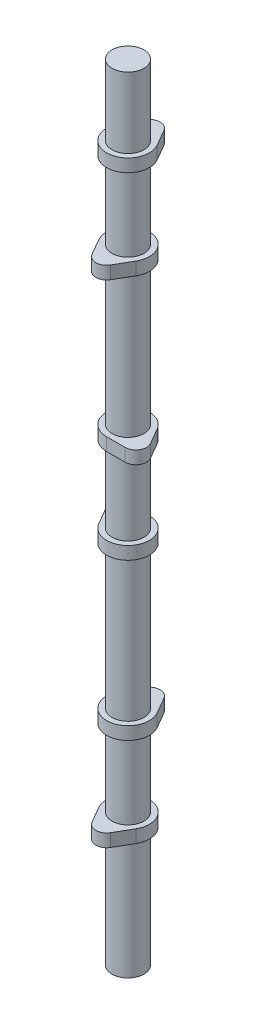
ISO-10303-21;
HEADER;
FILE_DESCRIPTION(('STEP AP214'),'2;1');
FILE_NAME('part.step','',(''),(''),'','','');
FILE_SCHEMA(('AUTOMOTIVE_DESIGN { 1 0 10303 214 1 1 1 1 }'));
ENDSEC;
DATA;
#1=APPLICATION_CONTEXT('core data for automotive mechanical design processes');
#2=APPLICATION_PROTOCOL_DEFINITION('international standard','automotive_design',2000,#1);
#3=PRODUCT_CONTEXT('',#1,'mechanical');
#4=PRODUCT('Part','Part','',(#3));
#5=PRODUCT_RELATED_PRODUCT_CATEGORY('part','',(#4));
#6=PRODUCT_DEFINITION_FORMATION('','',#4);
#7=PRODUCT_DEFINITION_CONTEXT('part definition',#1,'design');
#8=PRODUCT_DEFINITION('design','',#6,#7);
#9=PRODUCT_DEFINITION_SHAPE('','',#8);
#10=(LENGTH_UNIT() NAMED_UNIT(*) SI_UNIT(.MILLI.,.METRE.));
#11=(NAMED_UNIT(*) PLANE_ANGLE_UNIT() SI_UNIT($,.RADIAN.));
#12=(NAMED_UNIT(*) SI_UNIT($,.STERADIAN.) SOLID_ANGLE_UNIT());
#13=UNCERTAINTY_MEASURE_WITH_UNIT(LENGTH_MEASURE(1.E-05),#10,'distance_accuracy_value','');
#14=(GEOMETRIC_REPRESENTATION_CONTEXT(3) GLOBAL_UNCERTAINTY_ASSIGNED_CONTEXT((#13)) GLOBAL_UNIT_ASSIGNED_CONTEXT((#10,
#11,#12)) REPRESENTATION_CONTEXT('',''));
#15=CARTESIAN_POINT('',(0.,0.,0.));
#16=DIRECTION('',(0.,0.,1.));
#17=DIRECTION('',(1.,0.,0.));
#18=AXIS2_PLACEMENT_3D('',#15,#16,#17);
#19=CARTESIAN_POINT('',(0.,7.62,-12.7));
#20=DIRECTION('',(0.,-1.,0.));
#21=DIRECTION('',(0.,0.,-1.));
#22=AXIS2_PLACEMENT_3D('',#19,#20,#21);
#23=CYLINDRICAL_SURFACE('',#22,6.35);
#24=CARTESIAN_POINT('',(0.,0.,-12.7));
#25=DIRECTION('',(0.,1.,0.));
#26=DIRECTION('',(0.,0.,1.));
#27=AXIS2_PLACEMENT_3D('',#24,#25,#26);
#28=CIRCLE('',#27,6.35);
#29=CARTESIAN_POINT('',(5.49926131403118,0.,-15.875));
#30=VERTEX_POINT('',#29);
#31=CARTESIAN_POINT('',(-5.49926131403118,0.,-15.875));
#32=VERTEX_POINT('',#31);
#33=EDGE_CURVE('E384',#30,#32,#28,.T.);
#34=ORIENTED_EDGE('',*,*,#33,.T.);
#35=DIRECTION('',(0.,-1.,0.));
#36=VECTOR('',#35,1.);
#37=CARTESIAN_POINT('',(-5.49926131403118,7.62,-15.875));
#38=LINE('',#37,#36);
#39=CARTESIAN_POINT('',(-5.49926131403118,7.62,-15.875));
#40=VERTEX_POINT('',#39);
#41=EDGE_CURVE('E380',#40,#32,#38,.T.);
#42=ORIENTED_EDGE('',*,*,#41,.F.);
#43=CARTESIAN_POINT('',(0.,7.62,-12.7));
#44=DIRECTION('',(0.,1.,0.));
#45=DIRECTION('',(0.,0.,1.));
#46=AXIS2_PLACEMENT_3D('',#43,#44,#45);
#47=CIRCLE('',#46,6.35);
#48=CARTESIAN_POINT('',(5.49926131403118,7.62,-15.875));
#49=VERTEX_POINT('',#48);
#50=EDGE_CURVE('E378',#49,#40,#47,.T.);
#51=ORIENTED_EDGE('',*,*,#50,.F.);
#52=DIRECTION('',(0.,-1.,0.));
#53=VECTOR('',#52,1.);
#54=CARTESIAN_POINT('',(5.49926131403118,7.62,-15.875));
#55=LINE('',#54,#53);
#56=EDGE_CURVE('E383',#49,#30,#55,.T.);
#57=ORIENTED_EDGE('',*,*,#56,.T.);
#58=EDGE_LOOP('',(#34,#42,#51,#57));
#59=FACE_BOUND('',#58,.T.);
#60=ADVANCED_FACE('F39',(#59),#23,.T.);
#61=CARTESIAN_POINT('',(-5.49926131403118,7.62,-15.875));
#62=DIRECTION('',(0.866025403784438,0.,0.5));
#63=DIRECTION('',(0.5,0.,-0.866025403784439));
#64=AXIS2_PLACEMENT_3D('',#61,#62,#63);
#65=PLANE('',#64);
#66=DIRECTION('',(-0.5,0.,0.866025403784439));
#67=VECTOR('',#66,1.);
#68=CARTESIAN_POINT('',(-5.49926131403118,0.,-15.875));
#69=LINE('',#68,#67);
#70=CARTESIAN_POINT('',(-10.9985226280624,0.,-6.35));
#71=VERTEX_POINT('',#70);
#72=EDGE_CURVE('E389',#32,#71,#69,.T.);
#73=ORIENTED_EDGE('',*,*,#72,.T.);
#74=DIRECTION('',(0.,-1.,0.));
#75=VECTOR('',#74,1.);
#76=CARTESIAN_POINT('',(-10.9985226280624,7.62,-6.35));
#77=LINE('',#76,#75);
#78=CARTESIAN_POINT('',(-10.9985226280624,7.62,-6.35));
#79=VERTEX_POINT('',#78);
#80=EDGE_CURVE('E392',#79,#71,#77,.T.);
#81=ORIENTED_EDGE('',*,*,#80,.F.);
#82=DIRECTION('',(-0.5,0.,0.866025403784439));
#83=VECTOR('',#82,1.);
#84=CARTESIAN_POINT('',(-5.49926131403118,7.62,-15.875));
#85=LINE('',#84,#83);
#86=EDGE_CURVE('E87',#40,#79,#85,.T.);
#87=ORIENTED_EDGE('',*,*,#86,.F.);
#88=ORIENTED_EDGE('',*,*,#41,.T.);
#89=EDGE_LOOP('',(#73,#81,#87,#88));
#90=FACE_BOUND('',#89,.T.);
#91=ADVANCED_FACE('F464',(#90),#65,.F.);
#92=CARTESIAN_POINT('',(0.,7.62,0.));
#93=DIRECTION('',(0.,-1.,0.));
#94=DIRECTION('',(0.,0.,-1.));
#95=AXIS2_PLACEMENT_3D('',#92,#93,#94);
#96=CYLINDRICAL_SURFACE('',#95,12.7);
#97=CARTESIAN_POINT('',(0.,0.,0.));
#98=DIRECTION('',(0.,1.,0.));
#99=DIRECTION('',(0.,0.,1.));
#100=AXIS2_PLACEMENT_3D('',#97,#98,#99);
#101=CIRCLE('',#100,12.7);
#102=CARTESIAN_POINT('',(10.9985226280624,0.,-6.35));
#103=VERTEX_POINT('',#102);
#104=EDGE_CURVE('E71',#71,#103,#101,.T.);
#105=ORIENTED_EDGE('',*,*,#104,.T.);
#106=DIRECTION('',(0.,-1.,0.));
#107=VECTOR('',#106,1.);
#108=CARTESIAN_POINT('',(10.9985226280624,7.62,-6.35));
#109=LINE('',#108,#107);
#110=CARTESIAN_POINT('',(10.9985226280624,7.62,-6.35));
#111=VERTEX_POINT('',#110);
#112=EDGE_CURVE('E391',#111,#103,#109,.T.);
#113=ORIENTED_EDGE('',*,*,#112,.F.);
#114=CARTESIAN_POINT('',(0.,7.62,0.));
#115=DIRECTION('',(0.,1.,0.));
#116=DIRECTION('',(0.,0.,1.));
#117=AXIS2_PLACEMENT_3D('',#114,#115,#116);
#118=CIRCLE('',#117,12.7);
#119=EDGE_CURVE('E381',#79,#111,#118,.T.);
#120=ORIENTED_EDGE('',*,*,#119,.F.);
#121=ORIENTED_EDGE('',*,*,#80,.T.);
#122=EDGE_LOOP('',(#105,#113,#120,#121));
#123=FACE_BOUND('',#122,.T.);
#124=ADVANCED_FACE('F466',(#123),#96,.T.);
#125=CARTESIAN_POINT('',(5.49926131403118,7.62,-15.875));
#126=DIRECTION('',(-0.866025403784438,0.,0.5));
#127=DIRECTION('',(0.5,0.,0.866025403784439));
#128=AXIS2_PLACEMENT_3D('',#125,#126,#127);
#129=PLANE('',#128);
#130=DIRECTION('',(-0.5,0.,-0.866025403784439));
#131=VECTOR('',#130,1.);
#132=CARTESIAN_POINT('',(5.49926131403118,0.,-15.875));
#133=LINE('',#132,#131);
#134=EDGE_CURVE('E79',#103,#30,#133,.T.);
#135=ORIENTED_EDGE('',*,*,#134,.T.);
#136=ORIENTED_EDGE('',*,*,#56,.F.);
#137=DIRECTION('',(-0.5,0.,-0.866025403784439));
#138=VECTOR('',#137,1.);
#139=CARTESIAN_POINT('',(5.49926131403118,7.62,-15.875));
#140=LINE('',#139,#138);
#141=EDGE_CURVE('E54',#111,#49,#140,.T.);
#142=ORIENTED_EDGE('',*,*,#141,.F.);
#143=ORIENTED_EDGE('',*,*,#112,.T.);
#144=EDGE_LOOP('',(#135,#136,#142,#143));
#145=FACE_BOUND('',#144,.T.);
#146=ADVANCED_FACE('F476',(#145),#129,.F.);
#147=CARTESIAN_POINT('',(0.,7.62,-12.7));
#148=DIRECTION('',(0.,1.,0.));
#149=DIRECTION('',(0.,0.,1.));
#150=AXIS2_PLACEMENT_3D('',#147,#148,#149);
#151=PLANE('',#150);
#152=CARTESIAN_POINT('',(0.,7.62000000000002,0.));
#153=DIRECTION('',(0.,1.,0.));
#154=DIRECTION('',(0.,0.,1.));
#155=AXIS2_PLACEMENT_3D('',#152,#153,#154);
#156=CIRCLE('',#155,9.5);
#157=CARTESIAN_POINT('',(0.,7.62000000000002,9.5));
#158=VERTEX_POINT('',#157);
#159=EDGE_CURVE('E373',#158,#158,#156,.T.);
#160=ORIENTED_EDGE('',*,*,#159,.F.);
#161=EDGE_LOOP('',(#160));
#162=FACE_BOUND('',#161,.T.);
#163=ORIENTED_EDGE('',*,*,#50,.T.);
#164=ORIENTED_EDGE('',*,*,#86,.T.);
#165=ORIENTED_EDGE('',*,*,#119,.T.);
#166=ORIENTED_EDGE('',*,*,#141,.T.);
#167=EDGE_LOOP('',(#163,#164,#165,#166));
#168=FACE_BOUND('',#167,.T.);
#169=ADVANCED_FACE('F478',(#162,#168),#151,.T.);
#170=CARTESIAN_POINT('',(0.,0.,-12.7));
#171=DIRECTION('',(0.,1.,0.));
#172=DIRECTION('',(0.,0.,1.));
#173=AXIS2_PLACEMENT_3D('',#170,#171,#172);
#174=PLANE('',#173);
#175=CARTESIAN_POINT('',(0.,0.,0.));
#176=DIRECTION('',(0.,1.,0.));
#177=DIRECTION('',(0.,0.,1.));
#178=AXIS2_PLACEMENT_3D('',#175,#176,#177);
#179=CIRCLE('',#178,9.5);
#180=CARTESIAN_POINT('',(0.,0.,9.5));
#181=VERTEX_POINT('',#180);
#182=EDGE_CURVE('E369',#181,#181,#179,.T.);
#183=ORIENTED_EDGE('',*,*,#182,.T.);
#184=EDGE_LOOP('',(#183));
#185=FACE_BOUND('',#184,.T.);
#186=ORIENTED_EDGE('',*,*,#33,.F.);
#187=ORIENTED_EDGE('',*,*,#134,.F.);
#188=ORIENTED_EDGE('',*,*,#104,.F.);
#189=ORIENTED_EDGE('',*,*,#72,.F.);
#190=EDGE_LOOP('',(#186,#187,#188,#189));
#191=FACE_BOUND('',#190,.T.);
#192=ADVANCED_FACE('F475',(#185,#191),#174,.F.);
#193=CARTESIAN_POINT('',(0.,-416.56,0.));
#194=DIRECTION('',(0.,1.,0.));
#195=DIRECTION('',(0.,0.,1.));
#196=AXIS2_PLACEMENT_3D('',#193,#194,#195);
#197=CYLINDRICAL_SURFACE('',#196,9.5);
#198=CARTESIAN_POINT('',(0.,-45.72,0.));
#199=DIRECTION('',(0.,1.,0.));
#200=DIRECTION('',(0.,0.,1.));
#201=AXIS2_PLACEMENT_3D('',#198,#199,#200);
#202=CIRCLE('',#201,9.5);
#203=CARTESIAN_POINT('',(0.,-45.72,9.5));
#204=VERTEX_POINT('',#203);
#205=EDGE_CURVE('E376',#204,#204,#202,.F.);
#206=ORIENTED_EDGE('',*,*,#205,.F.);
#207=EDGE_LOOP('',(#206));
#208=FACE_BOUND('',#207,.T.);
#209=ORIENTED_EDGE('',*,*,#182,.F.);
#210=EDGE_LOOP('',(#209));
#211=FACE_BOUND('',#210,.T.);
#212=ADVANCED_FACE('F428',(#208,#211),#197,.T.);
#213=ORIENTED_EDGE('',*,*,#159,.T.);
#214=EDGE_LOOP('',(#213));
#215=FACE_BOUND('',#214,.T.);
#216=CARTESIAN_POINT('',(0.,49.53,0.));
#217=DIRECTION('',(0.,1.,0.));
#218=DIRECTION('',(0.,0.,1.));
#219=AXIS2_PLACEMENT_3D('',#216,#217,#218);
#220=CIRCLE('',#219,9.5);
#221=CARTESIAN_POINT('',(0.,49.53,9.5));
#222=VERTEX_POINT('',#221);
#223=EDGE_CURVE('E367',#222,#222,#220,.T.);
#224=ORIENTED_EDGE('',*,*,#223,.F.);
#225=EDGE_LOOP('',(#224));
#226=FACE_BOUND('',#225,.T.);
#227=ADVANCED_FACE('F487',(#215,#226),#197,.T.);
#228=CARTESIAN_POINT('',(0.,49.53,0.));
#229=DIRECTION('',(0.,1.,0.));
#230=DIRECTION('',(0.,0.,1.));
#231=AXIS2_PLACEMENT_3D('',#228,#229,#230);
#232=PLANE('',#231);
#233=ORIENTED_EDGE('',*,*,#223,.T.);
#234=EDGE_LOOP('',(#233));
#235=FACE_BOUND('',#234,.T.);
#236=ADVANCED_FACE('F525',(#235),#232,.T.);
#237=CARTESIAN_POINT('',(0.,-45.72,12.7));
#238=DIRECTION('',(0.,-1.,0.));
#239=DIRECTION('',(0.,0.,1.));
#240=AXIS2_PLACEMENT_3D('',#237,#238,#239);
#241=CYLINDRICAL_SURFACE('',#240,6.35);
#242=CARTESIAN_POINT('',(0.,-53.34,12.7));
#243=DIRECTION('',(0.,1.,0.));
#244=DIRECTION('',(0.,0.,-1.));
#245=AXIS2_PLACEMENT_3D('',#242,#243,#244);
#246=CIRCLE('',#245,6.35);
#247=CARTESIAN_POINT('',(-5.49926131403129,-53.34,15.875));
#248=VERTEX_POINT('',#247);
#249=CARTESIAN_POINT('',(5.49926131403107,-53.34,15.875));
#250=VERTEX_POINT('',#249);
#251=EDGE_CURVE('E347',#248,#250,#246,.T.);
#252=ORIENTED_EDGE('',*,*,#251,.T.);
#253=DIRECTION('',(0.,-1.,0.));
#254=VECTOR('',#253,1.);
#255=CARTESIAN_POINT('',(5.49926131403107,-45.72,15.875));
#256=LINE('',#255,#254);
#257=CARTESIAN_POINT('',(5.49926131403107,-45.72,15.875));
#258=VERTEX_POINT('',#257);
#259=EDGE_CURVE('E362',#258,#250,#256,.T.);
#260=ORIENTED_EDGE('',*,*,#259,.F.);
#261=CARTESIAN_POINT('',(0.,-45.72,12.7));
#262=DIRECTION('',(0.,1.,0.));
#263=DIRECTION('',(0.,0.,-1.));
#264=AXIS2_PLACEMENT_3D('',#261,#262,#263);
#265=CIRCLE('',#264,6.35);
#266=CARTESIAN_POINT('',(-5.49926131403129,-45.72,15.875));
#267=VERTEX_POINT('',#266);
#268=EDGE_CURVE('E333',#267,#258,#265,.T.);
#269=ORIENTED_EDGE('',*,*,#268,.F.);
#270=DIRECTION('',(0.,-1.,0.));
#271=VECTOR('',#270,1.);
#272=CARTESIAN_POINT('',(-5.49926131403129,-45.72,15.875));
#273=LINE('',#272,#271);
#274=EDGE_CURVE('E343',#267,#248,#273,.T.);
#275=ORIENTED_EDGE('',*,*,#274,.T.);
#276=EDGE_LOOP('',(#252,#260,#269,#275));
#277=FACE_BOUND('',#276,.T.);
#278=ADVANCED_FACE('F442',(#277),#241,.T.);
#279=CARTESIAN_POINT('',(5.49926131403107,-45.72,15.875));
#280=DIRECTION('',(-0.866025403784435,0.,-0.500000000000006));
#281=DIRECTION('',(-0.500000000000006,0.,0.866025403784435));
#282=AXIS2_PLACEMENT_3D('',#279,#280,#281);
#283=PLANE('',#282);
#284=DIRECTION('',(0.500000000000006,0.,-0.866025403784435));
#285=VECTOR('',#284,1.);
#286=CARTESIAN_POINT('',(5.49926131403107,-53.34,15.875));
#287=LINE('',#286,#285);
#288=CARTESIAN_POINT('',(10.9985226280623,-53.34,6.35000000000007));
#289=VERTEX_POINT('',#288);
#290=EDGE_CURVE('E349',#250,#289,#287,.T.);
#291=ORIENTED_EDGE('',*,*,#290,.T.);
#292=DIRECTION('',(0.,-1.,0.));
#293=VECTOR('',#292,1.);
#294=CARTESIAN_POINT('',(10.9985226280623,-45.72,6.35000000000007));
#295=LINE('',#294,#293);
#296=CARTESIAN_POINT('',(10.9985226280623,-45.72,6.35000000000007));
#297=VERTEX_POINT('',#296);
#298=EDGE_CURVE('E356',#297,#289,#295,.T.);
#299=ORIENTED_EDGE('',*,*,#298,.F.);
#300=DIRECTION('',(0.500000000000006,0.,-0.866025403784435));
#301=VECTOR('',#300,1.);
#302=CARTESIAN_POINT('',(5.49926131403107,-45.72,15.875));
#303=LINE('',#302,#301);
#304=EDGE_CURVE('E336',#258,#297,#303,.T.);
#305=ORIENTED_EDGE('',*,*,#304,.F.);
#306=ORIENTED_EDGE('',*,*,#259,.T.);
#307=EDGE_LOOP('',(#291,#299,#305,#306));
#308=FACE_BOUND('',#307,.T.);
#309=ADVANCED_FACE('F455',(#308),#283,.F.);
#310=CARTESIAN_POINT('',(0.,-45.72,0.));
#311=DIRECTION('',(0.,-1.,0.));
#312=DIRECTION('',(0.,0.,1.));
#313=AXIS2_PLACEMENT_3D('',#310,#311,#312);
#314=CYLINDRICAL_SURFACE('',#313,12.7);
#315=CARTESIAN_POINT('',(0.,-53.34,0.));
#316=DIRECTION('',(0.,1.,0.));
#317=DIRECTION('',(0.,0.,-1.));
#318=AXIS2_PLACEMENT_3D('',#315,#316,#317);
#319=CIRCLE('',#318,12.7);
#320=CARTESIAN_POINT('',(-10.9985226280624,-53.34,6.34999999999992));
#321=VERTEX_POINT('',#320);
#322=EDGE_CURVE('E353',#289,#321,#319,.T.);
#323=ORIENTED_EDGE('',*,*,#322,.T.);
#324=DIRECTION('',(0.,-1.,0.));
#325=VECTOR('',#324,1.);
#326=CARTESIAN_POINT('',(-10.9985226280624,-45.72,6.34999999999992));
#327=LINE('',#326,#325);
#328=CARTESIAN_POINT('',(-10.9985226280624,-45.72,6.34999999999992));
#329=VERTEX_POINT('',#328);
#330=EDGE_CURVE('E357',#329,#321,#327,.T.);
#331=ORIENTED_EDGE('',*,*,#330,.F.);
#332=CARTESIAN_POINT('',(0.,-45.72,0.));
#333=DIRECTION('',(0.,1.,0.));
#334=DIRECTION('',(0.,0.,-1.));
#335=AXIS2_PLACEMENT_3D('',#332,#333,#334);
#336=CIRCLE('',#335,12.7);
#337=EDGE_CURVE('E342',#297,#329,#336,.T.);
#338=ORIENTED_EDGE('',*,*,#337,.F.);
#339=ORIENTED_EDGE('',*,*,#298,.T.);
#340=EDGE_LOOP('',(#323,#331,#338,#339));
#341=FACE_BOUND('',#340,.T.);
#342=ADVANCED_FACE('F447',(#341),#314,.T.);
#343=CARTESIAN_POINT('',(-5.49926131403129,-45.72,15.875));
#344=DIRECTION('',(0.866025403784442,0.,-0.499999999999994));
#345=DIRECTION('',(-0.499999999999994,0.,-0.866025403784442));
#346=AXIS2_PLACEMENT_3D('',#343,#344,#345);
#347=PLANE('',#346);
#348=DIRECTION('',(0.499999999999994,0.,0.866025403784442));
#349=VECTOR('',#348,1.);
#350=CARTESIAN_POINT('',(-5.49926131403129,-53.34,15.875));
#351=LINE('',#350,#349);
#352=EDGE_CURVE('E339',#321,#248,#351,.T.);
#353=ORIENTED_EDGE('',*,*,#352,.T.);
#354=ORIENTED_EDGE('',*,*,#274,.F.);
#355=DIRECTION('',(0.499999999999994,0.,0.866025403784442));
#356=VECTOR('',#355,1.);
#357=CARTESIAN_POINT('',(-5.49926131403129,-45.72,15.875));
#358=LINE('',#357,#356);
#359=EDGE_CURVE('E345',#329,#267,#358,.T.);
#360=ORIENTED_EDGE('',*,*,#359,.F.);
#361=ORIENTED_EDGE('',*,*,#330,.T.);
#362=EDGE_LOOP('',(#353,#354,#360,#361));
#363=FACE_BOUND('',#362,.T.);
#364=ADVANCED_FACE('F448',(#363),#347,.F.);
#365=CARTESIAN_POINT('',(0.,-45.72,12.7));
#366=DIRECTION('',(0.,1.,0.));
#367=DIRECTION('',(0.,0.,-1.));
#368=AXIS2_PLACEMENT_3D('',#365,#366,#367);
#369=PLANE('',#368);
#370=ORIENTED_EDGE('',*,*,#205,.T.);
#371=EDGE_LOOP('',(#370));
#372=FACE_BOUND('',#371,.T.);
#373=ORIENTED_EDGE('',*,*,#268,.T.);
#374=ORIENTED_EDGE('',*,*,#304,.T.);
#375=ORIENTED_EDGE('',*,*,#337,.T.);
#376=ORIENTED_EDGE('',*,*,#359,.T.);
#377=EDGE_LOOP('',(#373,#374,#375,#376));
#378=FACE_BOUND('',#377,.T.);
#379=ADVANCED_FACE('F432',(#372,#378),#369,.T.);
#380=CARTESIAN_POINT('',(0.,-53.34,12.7));
#381=DIRECTION('',(0.,1.,0.));
#382=DIRECTION('',(0.,0.,-1.));
#383=AXIS2_PLACEMENT_3D('',#380,#381,#382);
#384=PLANE('',#383);
#385=CARTESIAN_POINT('',(0.,-53.34,0.));
#386=DIRECTION('',(0.,1.,0.));
#387=DIRECTION('',(0.,0.,1.));
#388=AXIS2_PLACEMENT_3D('',#385,#386,#387);
#389=CIRCLE('',#388,9.5);
#390=CARTESIAN_POINT('',(0.,-53.34,9.5));
#391=VERTEX_POINT('',#390);
#392=EDGE_CURVE('E364',#391,#391,#389,.F.);
#393=ORIENTED_EDGE('',*,*,#392,.F.);
#394=EDGE_LOOP('',(#393));
#395=FACE_BOUND('',#394,.T.);
#396=ORIENTED_EDGE('',*,*,#251,.F.);
#397=ORIENTED_EDGE('',*,*,#352,.F.);
#398=ORIENTED_EDGE('',*,*,#322,.F.);
#399=ORIENTED_EDGE('',*,*,#290,.F.);
#400=EDGE_LOOP('',(#396,#397,#398,#399));
#401=FACE_BOUND('',#400,.T.);
#402=ADVANCED_FACE('F426',(#395,#401),#384,.F.);
#403=CARTESIAN_POINT('',(0.,-138.43,0.));
#404=DIRECTION('',(0.,1.,0.));
#405=DIRECTION('',(0.,0.,1.));
#406=AXIS2_PLACEMENT_3D('',#403,#404,#405);
#407=CIRCLE('',#406,9.5);
#408=CARTESIAN_POINT('',(0.,-138.43,9.5));
#409=VERTEX_POINT('',#408);
#410=EDGE_CURVE('E50',#409,#409,#407,.F.);
#411=ORIENTED_EDGE('',*,*,#410,.F.);
#412=EDGE_LOOP('',(#411));
#413=FACE_BOUND('',#412,.T.);
#414=ORIENTED_EDGE('',*,*,#392,.T.);
#415=EDGE_LOOP('',(#414));
#416=FACE_BOUND('',#415,.T.);
#417=ADVANCED_FACE('F425',(#413,#416),#197,.T.);
#418=CARTESIAN_POINT('',(10.9985226280623,-138.43,6.35000000000005));
#419=DIRECTION('',(0.,-1.,0.));
#420=DIRECTION('',(0.866025403784436,0.,0.500000000000004));
#421=AXIS2_PLACEMENT_3D('',#418,#419,#420);
#422=CYLINDRICAL_SURFACE('',#421,6.35);
#423=CARTESIAN_POINT('',(10.9985226280623,-146.05,6.35000000000005));
#424=DIRECTION('',(0.,1.,0.));
#425=DIRECTION('',(-0.866025403784436,0.,-0.500000000000004));
#426=AXIS2_PLACEMENT_3D('',#423,#424,#425);
#427=CIRCLE('',#426,6.35);
#428=CARTESIAN_POINT('',(10.9985226280623,-146.05,12.7000000000001));
#429=VERTEX_POINT('',#428);
#430=CARTESIAN_POINT('',(16.4977839420935,-146.05,3.17500000000008));
#431=VERTEX_POINT('',#430);
#432=EDGE_CURVE('E236',#429,#431,#427,.T.);
#433=ORIENTED_EDGE('',*,*,#432,.T.);
#434=DIRECTION('',(0.,-1.,0.));
#435=VECTOR('',#434,1.);
#436=CARTESIAN_POINT('',(16.4977839420935,-138.43,3.17500000000008));
#437=LINE('',#436,#435);
#438=CARTESIAN_POINT('',(16.4977839420935,-138.43,3.17500000000008));
#439=VERTEX_POINT('',#438);
#440=EDGE_CURVE('E267',#439,#431,#437,.T.);
#441=ORIENTED_EDGE('',*,*,#440,.F.);
#442=CARTESIAN_POINT('',(10.9985226280623,-138.43,6.35000000000005));
#443=DIRECTION('',(0.,1.,0.));
#444=DIRECTION('',(-0.866025403784436,0.,-0.500000000000004));
#445=AXIS2_PLACEMENT_3D('',#442,#443,#444);
#446=CIRCLE('',#445,6.35);
#447=CARTESIAN_POINT('',(10.9985226280623,-138.43,12.7000000000001));
#448=VERTEX_POINT('',#447);
#449=EDGE_CURVE('E241',#448,#439,#446,.T.);
#450=ORIENTED_EDGE('',*,*,#449,.F.);
#451=DIRECTION('',(0.,-1.,0.));
#452=VECTOR('',#451,1.);
#453=CARTESIAN_POINT('',(10.9985226280623,-138.43,12.7000000000001));
#454=LINE('',#453,#452);
#455=EDGE_CURVE('E251',#448,#429,#454,.T.);
#456=ORIENTED_EDGE('',*,*,#455,.T.);
#457=EDGE_LOOP('',(#433,#441,#450,#456));
#458=FACE_BOUND('',#457,.T.);
#459=ADVANCED_FACE('F422',(#458),#422,.T.);
#460=CARTESIAN_POINT('',(16.4977839420935,-138.43,3.17500000000008));
#461=DIRECTION('',(-0.866025403784441,0.,0.499999999999996));
#462=DIRECTION('',(0.499999999999996,0.,0.866025403784441));
#463=AXIS2_PLACEMENT_3D('',#460,#461,#462);
#464=PLANE('',#463);
#465=DIRECTION('',(-0.499999999999996,0.,-0.866025403784441));
#466=VECTOR('',#465,1.);
#467=CARTESIAN_POINT('',(16.4977839420935,-146.05,3.17500000000008));
#468=LINE('',#467,#466);
#469=CARTESIAN_POINT('',(10.9985226280624,-146.05,-6.34999999999996));
#470=VERTEX_POINT('',#469);
#471=EDGE_CURVE('E258',#431,#470,#468,.T.);
#472=ORIENTED_EDGE('',*,*,#471,.T.);
#473=DIRECTION('',(0.,-1.,0.));
#474=VECTOR('',#473,1.);
#475=CARTESIAN_POINT('',(10.9985226280624,-138.43,-6.34999999999996));
#476=LINE('',#475,#474);
#477=CARTESIAN_POINT('',(10.9985226280624,-138.43,-6.34999999999996));
#478=VERTEX_POINT('',#477);
#479=EDGE_CURVE('E266',#478,#470,#476,.T.);
#480=ORIENTED_EDGE('',*,*,#479,.F.);
#481=DIRECTION('',(-0.499999999999996,0.,-0.866025403784441));
#482=VECTOR('',#481,1.);
#483=CARTESIAN_POINT('',(16.4977839420935,-138.43,3.17500000000008));
#484=LINE('',#483,#482);
#485=EDGE_CURVE('E247',#439,#478,#484,.T.);
#486=ORIENTED_EDGE('',*,*,#485,.F.);
#487=ORIENTED_EDGE('',*,*,#440,.T.);
#488=EDGE_LOOP('',(#472,#480,#486,#487));
#489=FACE_BOUND('',#488,.T.);
#490=ADVANCED_FACE('F671',(#489),#464,.F.);
#491=CARTESIAN_POINT('',(0.,-138.43,0.));
#492=DIRECTION('',(0.,-1.,0.));
#493=DIRECTION('',(0.866025403784436,0.,0.500000000000004));
#494=AXIS2_PLACEMENT_3D('',#491,#492,#493);
#495=CYLINDRICAL_SURFACE('',#494,12.7);
#496=CARTESIAN_POINT('',(0.,-146.05,0.));
#497=DIRECTION('',(0.,1.,0.));
#498=DIRECTION('',(-0.866025403784436,0.,-0.500000000000004));
#499=AXIS2_PLACEMENT_3D('',#496,#497,#498);
#500=CIRCLE('',#499,12.7);
#501=CARTESIAN_POINT('',(0.,-146.05,12.7));
#502=VERTEX_POINT('',#501);
#503=EDGE_CURVE('E256',#470,#502,#500,.T.);
#504=ORIENTED_EDGE('',*,*,#503,.T.);
#505=DIRECTION('',(0.,-1.,0.));
#506=VECTOR('',#505,1.);
#507=CARTESIAN_POINT('',(0.,-138.43,12.7));
#508=LINE('',#507,#506);
#509=CARTESIAN_POINT('',(0.,-138.43,12.7));
#510=VERTEX_POINT('',#509);
#511=EDGE_CURVE('E263',#510,#502,#508,.T.);
#512=ORIENTED_EDGE('',*,*,#511,.F.);
#513=CARTESIAN_POINT('',(0.,-138.43,0.));
#514=DIRECTION('',(0.,1.,0.));
#515=DIRECTION('',(-0.866025403784436,0.,-0.500000000000004));
#516=AXIS2_PLACEMENT_3D('',#513,#514,#515);
#517=CIRCLE('',#516,12.7);
#518=EDGE_CURVE('E246',#478,#510,#517,.T.);
#519=ORIENTED_EDGE('',*,*,#518,.F.);
#520=ORIENTED_EDGE('',*,*,#479,.T.);
#521=EDGE_LOOP('',(#504,#512,#519,#520));
#522=FACE_BOUND('',#521,.T.);
#523=ADVANCED_FACE('F684',(#522),#495,.T.);
#524=CARTESIAN_POINT('',(10.9985226280623,-138.43,12.7000000000001));
#525=DIRECTION('',(0.,0.,-1.));
#526=DIRECTION('',(-1.,0.,0.));
#527=AXIS2_PLACEMENT_3D('',#524,#525,#526);
#528=PLANE('',#527);
#529=DIRECTION('',(1.,0.,0.));
#530=VECTOR('',#529,1.);
#531=CARTESIAN_POINT('',(10.9985226280623,-146.05,12.7000000000001));
#532=LINE('',#531,#530);
#533=EDGE_CURVE('E249',#502,#429,#532,.T.);
#534=ORIENTED_EDGE('',*,*,#533,.T.);
#535=ORIENTED_EDGE('',*,*,#455,.F.);
#536=DIRECTION('',(1.,0.,0.));
#537=VECTOR('',#536,1.);
#538=CARTESIAN_POINT('',(10.9985226280623,-138.43,12.7000000000001));
#539=LINE('',#538,#537);
#540=EDGE_CURVE('E253',#510,#448,#539,.T.);
#541=ORIENTED_EDGE('',*,*,#540,.F.);
#542=ORIENTED_EDGE('',*,*,#511,.T.);
#543=EDGE_LOOP('',(#534,#535,#541,#542));
#544=FACE_BOUND('',#543,.T.);
#545=ADVANCED_FACE('F695',(#544),#528,.F.);
#546=CARTESIAN_POINT('',(10.9985226280623,-138.43,6.35000000000005));
#547=DIRECTION('',(0.,1.,0.));
#548=DIRECTION('',(-0.866025403784436,0.,-0.500000000000004));
#549=AXIS2_PLACEMENT_3D('',#546,#547,#548);
#550=PLANE('',#549);
#551=ORIENTED_EDGE('',*,*,#410,.T.);
#552=EDGE_LOOP('',(#551));
#553=FACE_BOUND('',#552,.T.);
#554=ORIENTED_EDGE('',*,*,#449,.T.);
#555=ORIENTED_EDGE('',*,*,#485,.T.);
#556=ORIENTED_EDGE('',*,*,#518,.T.);
#557=ORIENTED_EDGE('',*,*,#540,.T.);
#558=EDGE_LOOP('',(#554,#555,#556,#557));
#559=FACE_BOUND('',#558,.T.);
#560=ADVANCED_FACE('F420',(#553,#559),#550,.T.);
#561=CARTESIAN_POINT('',(10.9985226280623,-146.05,6.35000000000005));
#562=DIRECTION('',(0.,1.,0.));
#563=DIRECTION('',(-0.866025403784436,0.,-0.500000000000004));
#564=AXIS2_PLACEMENT_3D('',#561,#562,#563);
#565=PLANE('',#564);
#566=CARTESIAN_POINT('',(0.,-146.05,0.));
#567=DIRECTION('',(0.,1.,0.));
#568=DIRECTION('',(0.,0.,1.));
#569=AXIS2_PLACEMENT_3D('',#566,#567,#568);
#570=CIRCLE('',#569,9.5);
#571=CARTESIAN_POINT('',(0.,-146.05,9.5));
#572=VERTEX_POINT('',#571);
#573=EDGE_CURVE('E275',#572,#572,#570,.F.);
#574=ORIENTED_EDGE('',*,*,#573,.F.);
#575=EDGE_LOOP('',(#574));
#576=FACE_BOUND('',#575,.T.);
#577=ORIENTED_EDGE('',*,*,#432,.F.);
#578=ORIENTED_EDGE('',*,*,#533,.F.);
#579=ORIENTED_EDGE('',*,*,#503,.F.);
#580=ORIENTED_EDGE('',*,*,#471,.F.);
#581=EDGE_LOOP('',(#577,#578,#579,#580));
#582=FACE_BOUND('',#581,.T.);
#583=ADVANCED_FACE('F712',(#576,#582),#565,.F.);
#584=CARTESIAN_POINT('',(0.,-191.77,0.));
#585=DIRECTION('',(0.,1.,0.));
#586=DIRECTION('',(0.,0.,1.));
#587=AXIS2_PLACEMENT_3D('',#584,#585,#586);
#588=CIRCLE('',#587,9.5);
#589=CARTESIAN_POINT('',(0.,-191.77,9.5));
#590=VERTEX_POINT('',#589);
#591=EDGE_CURVE('E11',#590,#590,#588,.F.);
#592=ORIENTED_EDGE('',*,*,#591,.F.);
#593=EDGE_LOOP('',(#592));
#594=FACE_BOUND('',#593,.T.);
#595=ORIENTED_EDGE('',*,*,#573,.T.);
#596=EDGE_LOOP('',(#595));
#597=FACE_BOUND('',#596,.T.);
#598=ADVANCED_FACE('F725',(#594,#597),#197,.T.);
#599=CARTESIAN_POINT('',(-10.9985226280623,-191.77,-6.35000000000013));
#600=DIRECTION('',(0.,-1.,0.));
#601=DIRECTION('',(-0.866025403784433,0.,-0.50000000000001));
#602=AXIS2_PLACEMENT_3D('',#599,#600,#601);
#603=CYLINDRICAL_SURFACE('',#602,6.35);
#604=CARTESIAN_POINT('',(-10.9985226280623,-199.39,-6.35000000000013));
#605=DIRECTION('',(0.,1.,0.));
#606=DIRECTION('',(0.866025403784433,0.,0.50000000000001));
#607=AXIS2_PLACEMENT_3D('',#604,#605,#606);
#608=CIRCLE('',#607,6.35);
#609=CARTESIAN_POINT('',(-10.9985226280622,-199.39,-12.7000000000001));
#610=VERTEX_POINT('',#609);
#611=CARTESIAN_POINT('',(-16.4977839420935,-199.39,-3.17500000000019));
#612=VERTEX_POINT('',#611);
#613=EDGE_CURVE('E231',#610,#612,#608,.T.);
#614=ORIENTED_EDGE('',*,*,#613,.T.);
#615=DIRECTION('',(0.,-1.,0.));
#616=VECTOR('',#615,1.);
#617=CARTESIAN_POINT('',(-16.4977839420935,-191.77,-3.17500000000019));
#618=LINE('',#617,#616);
#619=CARTESIAN_POINT('',(-16.4977839420935,-191.77,-3.17500000000019));
#620=VERTEX_POINT('',#619);
#621=EDGE_CURVE('E212',#620,#612,#618,.T.);
#622=ORIENTED_EDGE('',*,*,#621,.F.);
#623=CARTESIAN_POINT('',(-10.9985226280623,-191.77,-6.35000000000013));
#624=DIRECTION('',(0.,1.,0.));
#625=DIRECTION('',(0.866025403784433,0.,0.50000000000001));
#626=AXIS2_PLACEMENT_3D('',#623,#624,#625);
#627=CIRCLE('',#626,6.35);
#628=CARTESIAN_POINT('',(-10.9985226280622,-191.77,-12.7000000000001));
#629=VERTEX_POINT('',#628);
#630=EDGE_CURVE('E222',#629,#620,#627,.T.);
#631=ORIENTED_EDGE('',*,*,#630,.F.);
#632=DIRECTION('',(0.,-1.,0.));
#633=VECTOR('',#632,1.);
#634=CARTESIAN_POINT('',(-10.9985226280622,-191.77,-12.7000000000001));
#635=LINE('',#634,#633);
#636=EDGE_CURVE('E875',#629,#610,#635,.T.);
#637=ORIENTED_EDGE('',*,*,#636,.T.);
#638=EDGE_LOOP('',(#614,#622,#631,#637));
#639=FACE_BOUND('',#638,.T.);
#640=ADVANCED_FACE('F234',(#639),#603,.T.);
#641=CARTESIAN_POINT('',(-16.4977839420935,-191.77,-3.17500000000019));
#642=DIRECTION('',(0.866025403784445,0.,-0.49999999999999));
#643=DIRECTION('',(-0.49999999999999,0.,-0.866025403784445));
#644=AXIS2_PLACEMENT_3D('',#641,#642,#643);
#645=PLANE('',#644);
#646=DIRECTION('',(0.49999999999999,0.,0.866025403784445));
#647=VECTOR('',#646,1.);
#648=CARTESIAN_POINT('',(-16.4977839420935,-199.39,-3.17500000000019));
#649=LINE('',#648,#647);
#650=CARTESIAN_POINT('',(-10.9985226280624,-199.39,6.34999999999988));
#651=VERTEX_POINT('',#650);
#652=EDGE_CURVE('E861',#612,#651,#649,.T.);
#653=ORIENTED_EDGE('',*,*,#652,.T.);
#654=DIRECTION('',(0.,-1.,0.));
#655=VECTOR('',#654,1.);
#656=CARTESIAN_POINT('',(-10.9985226280624,-191.77,6.34999999999988));
#657=LINE('',#656,#655);
#658=CARTESIAN_POINT('',(-10.9985226280624,-191.77,6.34999999999988));
#659=VERTEX_POINT('',#658);
#660=EDGE_CURVE('E220',#659,#651,#657,.T.);
#661=ORIENTED_EDGE('',*,*,#660,.F.);
#662=DIRECTION('',(0.49999999999999,0.,0.866025403784445));
#663=VECTOR('',#662,1.);
#664=CARTESIAN_POINT('',(-16.4977839420935,-191.77,-3.17500000000019));
#665=LINE('',#664,#663);
#666=EDGE_CURVE('E209',#620,#659,#665,.T.);
#667=ORIENTED_EDGE('',*,*,#666,.F.);
#668=ORIENTED_EDGE('',*,*,#621,.T.);
#669=EDGE_LOOP('',(#653,#661,#667,#668));
#670=FACE_BOUND('',#669,.T.);
#671=ADVANCED_FACE('F215',(#670),#645,.F.);
#672=CARTESIAN_POINT('',(0.,-191.77,0.));
#673=DIRECTION('',(0.,-1.,0.));
#674=DIRECTION('',(-0.866025403784433,0.,-0.50000000000001));
#675=AXIS2_PLACEMENT_3D('',#672,#673,#674);
#676=CYLINDRICAL_SURFACE('',#675,12.7);
#677=CARTESIAN_POINT('',(0.,-199.39,0.));
#678=DIRECTION('',(0.,1.,0.));
#679=DIRECTION('',(0.866025403784433,0.,0.50000000000001));
#680=AXIS2_PLACEMENT_3D('',#677,#678,#679);
#681=CIRCLE('',#680,12.7);
#682=CARTESIAN_POINT('',(1.48318857196017E-13,-199.39,-12.7));
#683=VERTEX_POINT('',#682);
#684=EDGE_CURVE('E862',#651,#683,#681,.T.);
#685=ORIENTED_EDGE('',*,*,#684,.T.);
#686=DIRECTION('',(0.,-1.,0.));
#687=VECTOR('',#686,1.);
#688=CARTESIAN_POINT('',(1.48318857196017E-13,-191.77,-12.7));
#689=LINE('',#688,#687);
#690=CARTESIAN_POINT('',(1.48318857196017E-13,-191.77,-12.7));
#691=VERTEX_POINT('',#690);
#692=EDGE_CURVE('E239',#691,#683,#689,.T.);
#693=ORIENTED_EDGE('',*,*,#692,.F.);
#694=CARTESIAN_POINT('',(0.,-191.77,0.));
#695=DIRECTION('',(0.,1.,0.));
#696=DIRECTION('',(0.866025403784433,0.,0.50000000000001));
#697=AXIS2_PLACEMENT_3D('',#694,#695,#696);
#698=CIRCLE('',#697,12.7);
#699=EDGE_CURVE('E219',#659,#691,#698,.T.);
#700=ORIENTED_EDGE('',*,*,#699,.F.);
#701=ORIENTED_EDGE('',*,*,#660,.T.);
#702=EDGE_LOOP('',(#685,#693,#700,#701));
#703=FACE_BOUND('',#702,.T.);
#704=ADVANCED_FACE('F742',(#703),#676,.T.);
#705=CARTESIAN_POINT('',(-10.9985226280622,-191.77,-12.7000000000001));
#706=DIRECTION('',(0.,0.,1.));
#707=DIRECTION('',(1.,0.,0.));
#708=AXIS2_PLACEMENT_3D('',#705,#706,#707);
#709=PLANE('',#708);
#710=DIRECTION('',(-1.,0.,0.));
#711=VECTOR('',#710,1.);
#712=CARTESIAN_POINT('',(-10.9985226280622,-199.39,-12.7000000000001));
#713=LINE('',#712,#711);
#714=EDGE_CURVE('E227',#683,#610,#713,.T.);
#715=ORIENTED_EDGE('',*,*,#714,.T.);
#716=ORIENTED_EDGE('',*,*,#636,.F.);
#717=DIRECTION('',(-1.,0.,0.));
#718=VECTOR('',#717,1.);
#719=CARTESIAN_POINT('',(-10.9985226280622,-191.77,-12.7000000000001));
#720=LINE('',#719,#718);
#721=EDGE_CURVE('E228',#691,#629,#720,.T.);
#722=ORIENTED_EDGE('',*,*,#721,.F.);
#723=ORIENTED_EDGE('',*,*,#692,.T.);
#724=EDGE_LOOP('',(#715,#716,#722,#723));
#725=FACE_BOUND('',#724,.T.);
#726=ADVANCED_FACE('F749',(#725),#709,.F.);
#727=CARTESIAN_POINT('',(-10.9985226280623,-191.77,-6.35000000000013));
#728=DIRECTION('',(0.,1.,0.));
#729=DIRECTION('',(0.866025403784433,0.,0.50000000000001));
#730=AXIS2_PLACEMENT_3D('',#727,#728,#729);
#731=PLANE('',#730);
#732=ORIENTED_EDGE('',*,*,#591,.T.);
#733=EDGE_LOOP('',(#732));
#734=FACE_BOUND('',#733,.T.);
#735=ORIENTED_EDGE('',*,*,#630,.T.);
#736=ORIENTED_EDGE('',*,*,#666,.T.);
#737=ORIENTED_EDGE('',*,*,#699,.T.);
#738=ORIENTED_EDGE('',*,*,#721,.T.);
#739=EDGE_LOOP('',(#735,#736,#737,#738));
#740=FACE_BOUND('',#739,.T.);
#741=ADVANCED_FACE('F221',(#734,#740),#731,.T.);
#742=CARTESIAN_POINT('',(-10.9985226280623,-199.39,-6.35000000000013));
#743=DIRECTION('',(0.,1.,0.));
#744=DIRECTION('',(0.866025403784433,0.,0.50000000000001));
#745=AXIS2_PLACEMENT_3D('',#742,#743,#744);
#746=PLANE('',#745);
#747=CARTESIAN_POINT('',(0.,-199.39,0.));
#748=DIRECTION('',(0.,1.,0.));
#749=DIRECTION('',(0.,0.,1.));
#750=AXIS2_PLACEMENT_3D('',#747,#748,#749);
#751=CIRCLE('',#750,9.5);
#752=CARTESIAN_POINT('',(0.,-199.39,9.5));
#753=VERTEX_POINT('',#752);
#754=EDGE_CURVE('E233',#753,#753,#751,.F.);
#755=ORIENTED_EDGE('',*,*,#754,.F.);
#756=EDGE_LOOP('',(#755));
#757=FACE_BOUND('',#756,.T.);
#758=ORIENTED_EDGE('',*,*,#613,.F.);
#759=ORIENTED_EDGE('',*,*,#714,.F.);
#760=ORIENTED_EDGE('',*,*,#684,.F.);
#761=ORIENTED_EDGE('',*,*,#652,.F.);
#762=EDGE_LOOP('',(#758,#759,#760,#761));
#763=FACE_BOUND('',#762,.T.);
#764=ADVANCED_FACE('F768',(#757,#763),#746,.F.);
#765=CARTESIAN_POINT('',(0.,-416.56,0.));
#766=DIRECTION('',(0.,1.,0.));
#767=DIRECTION('',(0.,0.,1.));
#768=AXIS2_PLACEMENT_3D('',#765,#766,#767);
#769=PLANE('',#768);
#770=CARTESIAN_POINT('',(0.,-416.56,0.));
#771=DIRECTION('',(0.,1.,0.));
#772=DIRECTION('',(0.,0.,1.));
#773=AXIS2_PLACEMENT_3D('',#770,#771,#772);
#774=CIRCLE('',#773,9.5);
#775=CARTESIAN_POINT('',(0.,-416.56,9.5));
#776=VERTEX_POINT('',#775);
#777=EDGE_CURVE('E368',#776,#776,#774,.T.);
#778=ORIENTED_EDGE('',*,*,#777,.F.);
#779=EDGE_LOOP('',(#778));
#780=FACE_BOUND('',#779,.T.);
#781=ADVANCED_FACE('F779',(#780),#769,.F.);
#782=ORIENTED_EDGE('',*,*,#777,.T.);
#783=EDGE_LOOP('',(#782));
#784=FACE_BOUND('',#783,.T.);
#785=CARTESIAN_POINT('',(0.,-345.44,0.));
#786=DIRECTION('',(0.,1.,0.));
#787=DIRECTION('',(0.,0.,1.));
#788=AXIS2_PLACEMENT_3D('',#785,#786,#787);
#789=CIRCLE('',#788,9.5);
#790=CARTESIAN_POINT('',(0.,-345.44,9.5));
#791=VERTEX_POINT('',#790);
#792=EDGE_CURVE('E305',#791,#791,#789,.F.);
#793=ORIENTED_EDGE('',*,*,#792,.T.);
#794=EDGE_LOOP('',(#793));
#795=FACE_BOUND('',#794,.T.);
#796=ADVANCED_FACE('F663',(#784,#795),#197,.T.);
#797=CARTESIAN_POINT('',(0.,-345.44,12.7));
#798=DIRECTION('',(0.,1.,0.));
#799=DIRECTION('',(0.,0.,-1.));
#800=AXIS2_PLACEMENT_3D('',#797,#798,#799);
#801=PLANE('',#800);
#802=ORIENTED_EDGE('',*,*,#792,.F.);
#803=EDGE_LOOP('',(#802));
#804=FACE_BOUND('',#803,.T.);
#805=CARTESIAN_POINT('',(0.,-345.44,12.7));
#806=DIRECTION('',(0.,1.,0.));
#807=DIRECTION('',(0.,0.,-1.));
#808=AXIS2_PLACEMENT_3D('',#805,#806,#807);
#809=CIRCLE('',#808,6.35);
#810=CARTESIAN_POINT('',(-5.49926131403129,-345.44,15.875));
#811=VERTEX_POINT('',#810);
#812=CARTESIAN_POINT('',(5.49926131403107,-345.44,15.875));
#813=VERTEX_POINT('',#812);
#814=EDGE_CURVE('E284',#811,#813,#809,.T.);
#815=ORIENTED_EDGE('',*,*,#814,.F.);
#816=DIRECTION('',(0.499999999999994,0.,0.866025403784442));
#817=VECTOR('',#816,1.);
#818=CARTESIAN_POINT('',(-5.49926131403129,-345.44,15.875));
#819=LINE('',#818,#817);
#820=CARTESIAN_POINT('',(-10.9985226280624,-345.44,6.34999999999992));
#821=VERTEX_POINT('',#820);
#822=EDGE_CURVE('E280',#821,#811,#819,.T.);
#823=ORIENTED_EDGE('',*,*,#822,.F.);
#824=CARTESIAN_POINT('',(0.,-345.44,0.));
#825=DIRECTION('',(0.,1.,0.));
#826=DIRECTION('',(0.,0.,-1.));
#827=AXIS2_PLACEMENT_3D('',#824,#825,#826);
#828=CIRCLE('',#827,12.7);
#829=CARTESIAN_POINT('',(10.9985226280623,-345.44,6.35000000000007));
#830=VERTEX_POINT('',#829);
#831=EDGE_CURVE('E286',#830,#821,#828,.T.);
#832=ORIENTED_EDGE('',*,*,#831,.F.);
#833=DIRECTION('',(0.500000000000006,0.,-0.866025403784435));
#834=VECTOR('',#833,1.);
#835=CARTESIAN_POINT('',(5.49926131403107,-345.44,15.875));
#836=LINE('',#835,#834);
#837=EDGE_CURVE('E289',#813,#830,#836,.T.);
#838=ORIENTED_EDGE('',*,*,#837,.F.);
#839=EDGE_LOOP('',(#815,#823,#832,#838));
#840=FACE_BOUND('',#839,.T.);
#841=ADVANCED_FACE('F648',(#804,#840),#801,.F.);
#842=CARTESIAN_POINT('',(-5.49926131403129,-337.82,15.875));
#843=DIRECTION('',(0.866025403784442,0.,-0.499999999999994));
#844=DIRECTION('',(-0.499999999999994,0.,-0.866025403784442));
#845=AXIS2_PLACEMENT_3D('',#842,#843,#844);
#846=PLANE('',#845);
#847=ORIENTED_EDGE('',*,*,#822,.T.);
#848=DIRECTION('',(0.,-1.,0.));
#849=VECTOR('',#848,1.);
#850=CARTESIAN_POINT('',(-5.49926131403129,-337.82,15.875));
#851=LINE('',#850,#849);
#852=CARTESIAN_POINT('',(-5.49926131403129,-337.82,15.875));
#853=VERTEX_POINT('',#852);
#854=EDGE_CURVE('E281',#853,#811,#851,.T.);
#855=ORIENTED_EDGE('',*,*,#854,.F.);
#856=DIRECTION('',(0.499999999999994,0.,0.866025403784442));
#857=VECTOR('',#856,1.);
#858=CARTESIAN_POINT('',(-5.49926131403129,-337.82,15.875));
#859=LINE('',#858,#857);
#860=CARTESIAN_POINT('',(-10.9985226280624,-337.82,6.34999999999992));
#861=VERTEX_POINT('',#860);
#862=EDGE_CURVE('E283',#861,#853,#859,.T.);
#863=ORIENTED_EDGE('',*,*,#862,.F.);
#864=DIRECTION('',(0.,-1.,0.));
#865=VECTOR('',#864,1.);
#866=CARTESIAN_POINT('',(-10.9985226280624,-337.82,6.34999999999992));
#867=LINE('',#866,#865);
#868=EDGE_CURVE('E294',#861,#821,#867,.T.);
#869=ORIENTED_EDGE('',*,*,#868,.T.);
#870=EDGE_LOOP('',(#847,#855,#863,#869));
#871=FACE_BOUND('',#870,.T.);
#872=ADVANCED_FACE('F640',(#871),#846,.F.);
#873=CARTESIAN_POINT('',(0.,-337.82,0.));
#874=DIRECTION('',(0.,-1.,0.));
#875=DIRECTION('',(0.,0.,1.));
#876=AXIS2_PLACEMENT_3D('',#873,#874,#875);
#877=CYLINDRICAL_SURFACE('',#876,12.7);
#878=ORIENTED_EDGE('',*,*,#831,.T.);
#879=ORIENTED_EDGE('',*,*,#868,.F.);
#880=CARTESIAN_POINT('',(0.,-337.82,0.));
#881=DIRECTION('',(0.,1.,0.));
#882=DIRECTION('',(0.,0.,-1.));
#883=AXIS2_PLACEMENT_3D('',#880,#881,#882);
#884=CIRCLE('',#883,12.7);
#885=CARTESIAN_POINT('',(10.9985226280623,-337.82,6.35000000000007));
#886=VERTEX_POINT('',#885);
#887=EDGE_CURVE('E276',#886,#861,#884,.T.);
#888=ORIENTED_EDGE('',*,*,#887,.F.);
#889=DIRECTION('',(0.,-1.,0.));
#890=VECTOR('',#889,1.);
#891=CARTESIAN_POINT('',(10.9985226280623,-337.82,6.35000000000007));
#892=LINE('',#891,#890);
#893=EDGE_CURVE('E300',#886,#830,#892,.T.);
#894=ORIENTED_EDGE('',*,*,#893,.T.);
#895=EDGE_LOOP('',(#878,#879,#888,#894));
#896=FACE_BOUND('',#895,.T.);
#897=ADVANCED_FACE('F627',(#896),#877,.T.);
#898=CARTESIAN_POINT('',(5.49926131403107,-337.82,15.875));
#899=DIRECTION('',(-0.866025403784435,0.,-0.500000000000006));
#900=DIRECTION('',(-0.500000000000006,0.,0.866025403784435));
#901=AXIS2_PLACEMENT_3D('',#898,#899,#900);
#902=PLANE('',#901);
#903=ORIENTED_EDGE('',*,*,#837,.T.);
#904=ORIENTED_EDGE('',*,*,#893,.F.);
#905=DIRECTION('',(0.500000000000006,0.,-0.866025403784435));
#906=VECTOR('',#905,1.);
#907=CARTESIAN_POINT('',(5.49926131403107,-337.82,15.875));
#908=LINE('',#907,#906);
#909=CARTESIAN_POINT('',(5.49926131403107,-337.82,15.875));
#910=VERTEX_POINT('',#909);
#911=EDGE_CURVE('E277',#910,#886,#908,.T.);
#912=ORIENTED_EDGE('',*,*,#911,.F.);
#913=DIRECTION('',(0.,-1.,0.));
#914=VECTOR('',#913,1.);
#915=CARTESIAN_POINT('',(5.49926131403107,-337.82,15.875));
#916=LINE('',#915,#914);
#917=EDGE_CURVE('E297',#910,#813,#916,.T.);
#918=ORIENTED_EDGE('',*,*,#917,.T.);
#919=EDGE_LOOP('',(#903,#904,#912,#918));
#920=FACE_BOUND('',#919,.T.);
#921=ADVANCED_FACE('F622',(#920),#902,.F.);
#922=CARTESIAN_POINT('',(0.,-337.82,12.7));
#923=DIRECTION('',(0.,-1.,0.));
#924=DIRECTION('',(0.,0.,1.));
#925=AXIS2_PLACEMENT_3D('',#922,#923,#924);
#926=CYLINDRICAL_SURFACE('',#925,6.35);
#927=ORIENTED_EDGE('',*,*,#814,.T.);
#928=ORIENTED_EDGE('',*,*,#917,.F.);
#929=CARTESIAN_POINT('',(0.,-337.82,12.7));
#930=DIRECTION('',(0.,1.,0.));
#931=DIRECTION('',(0.,0.,-1.));
#932=AXIS2_PLACEMENT_3D('',#929,#930,#931);
#933=CIRCLE('',#932,6.35);
#934=EDGE_CURVE('E272',#853,#910,#933,.T.);
#935=ORIENTED_EDGE('',*,*,#934,.F.);
#936=ORIENTED_EDGE('',*,*,#854,.T.);
#937=EDGE_LOOP('',(#927,#928,#935,#936));
#938=FACE_BOUND('',#937,.T.);
#939=ADVANCED_FACE('F612',(#938),#926,.T.);
#940=CARTESIAN_POINT('',(0.,-337.82,12.7));
#941=DIRECTION('',(0.,1.,0.));
#942=DIRECTION('',(0.,0.,-1.));
#943=AXIS2_PLACEMENT_3D('',#940,#941,#942);
#944=PLANE('',#943);
#945=CARTESIAN_POINT('',(0.,-337.82,0.));
#946=DIRECTION('',(0.,1.,0.));
#947=DIRECTION('',(0.,0.,1.));
#948=AXIS2_PLACEMENT_3D('',#945,#946,#947);
#949=CIRCLE('',#948,9.5);
#950=CARTESIAN_POINT('',(0.,-337.82,9.5));
#951=VERTEX_POINT('',#950);
#952=EDGE_CURVE('E409',#951,#951,#949,.F.);
#953=ORIENTED_EDGE('',*,*,#952,.T.);
#954=EDGE_LOOP('',(#953));
#955=FACE_BOUND('',#954,.T.);
#956=ORIENTED_EDGE('',*,*,#934,.T.);
#957=ORIENTED_EDGE('',*,*,#911,.T.);
#958=ORIENTED_EDGE('',*,*,#887,.T.);
#959=ORIENTED_EDGE('',*,*,#862,.T.);
#960=EDGE_LOOP('',(#956,#957,#958,#959));
#961=FACE_BOUND('',#960,.T.);
#962=ADVANCED_FACE('F618',(#955,#961),#944,.T.);
#963=ORIENTED_EDGE('',*,*,#952,.F.);
#964=EDGE_LOOP('',(#963));
#965=FACE_BOUND('',#964,.T.);
#966=CARTESIAN_POINT('',(0.,-292.1,0.));
#967=DIRECTION('',(0.,1.,0.));
#968=DIRECTION('',(0.,0.,1.));
#969=AXIS2_PLACEMENT_3D('',#966,#967,#968);
#970=CIRCLE('',#969,9.5);
#971=CARTESIAN_POINT('',(0.,-292.1,9.5));
#972=VERTEX_POINT('',#971);
#973=EDGE_CURVE('E331',#972,#972,#970,.F.);
#974=ORIENTED_EDGE('',*,*,#973,.T.);
#975=EDGE_LOOP('',(#974));
#976=FACE_BOUND('',#975,.T.);
#977=ADVANCED_FACE('F427',(#965,#976),#197,.T.);
#978=CARTESIAN_POINT('',(0.,-292.1,-12.7));
#979=DIRECTION('',(0.,1.,0.));
#980=DIRECTION('',(0.,0.,1.));
#981=AXIS2_PLACEMENT_3D('',#978,#979,#980);
#982=PLANE('',#981);
#983=ORIENTED_EDGE('',*,*,#973,.F.);
#984=EDGE_LOOP('',(#983));
#985=FACE_BOUND('',#984,.T.);
#986=CARTESIAN_POINT('',(0.,-292.1,-12.7));
#987=DIRECTION('',(0.,1.,0.));
#988=DIRECTION('',(0.,0.,1.));
#989=AXIS2_PLACEMENT_3D('',#986,#987,#988);
#990=CIRCLE('',#989,6.35);
#991=CARTESIAN_POINT('',(5.49926131403118,-292.1,-15.875));
#992=VERTEX_POINT('',#991);
#993=CARTESIAN_POINT('',(-5.49926131403118,-292.1,-15.875));
#994=VERTEX_POINT('',#993);
#995=EDGE_CURVE('E312',#992,#994,#990,.T.);
#996=ORIENTED_EDGE('',*,*,#995,.F.);
#997=DIRECTION('',(-0.5,0.,-0.866025403784439));
#998=VECTOR('',#997,1.);
#999=CARTESIAN_POINT('',(5.49926131403118,-292.1,-15.875));
#1000=LINE('',#999,#998);
#1001=CARTESIAN_POINT('',(10.9985226280624,-292.1,-6.35));
#1002=VERTEX_POINT('',#1001);
#1003=EDGE_CURVE('E306',#1002,#992,#1000,.T.);
#1004=ORIENTED_EDGE('',*,*,#1003,.F.);
#1005=CARTESIAN_POINT('',(0.,-292.1,0.));
#1006=DIRECTION('',(0.,1.,0.));
#1007=DIRECTION('',(0.,0.,1.));
#1008=AXIS2_PLACEMENT_3D('',#1005,#1006,#1007);
#1009=CIRCLE('',#1008,12.7);
#1010=CARTESIAN_POINT('',(-10.9985226280624,-292.1,-6.35));
#1011=VERTEX_POINT('',#1010);
#1012=EDGE_CURVE('E319',#1011,#1002,#1009,.T.);
#1013=ORIENTED_EDGE('',*,*,#1012,.F.);
#1014=DIRECTION('',(-0.5,0.,0.866025403784439));
#1015=VECTOR('',#1014,1.);
#1016=CARTESIAN_POINT('',(-5.49926131403118,-292.1,-15.875));
#1017=LINE('',#1016,#1015);
#1018=EDGE_CURVE('E318',#994,#1011,#1017,.T.);
#1019=ORIENTED_EDGE('',*,*,#1018,.F.);
#1020=EDGE_LOOP('',(#996,#1004,#1013,#1019));
#1021=FACE_BOUND('',#1020,.T.);
#1022=ADVANCED_FACE('F593',(#985,#1021),#982,.F.);
#1023=CARTESIAN_POINT('',(5.49926131403118,-284.48,-15.875));
#1024=DIRECTION('',(-0.866025403784438,0.,0.5));
#1025=DIRECTION('',(0.5,0.,0.866025403784439));
#1026=AXIS2_PLACEMENT_3D('',#1023,#1024,#1025);
#1027=PLANE('',#1026);
#1028=ORIENTED_EDGE('',*,*,#1003,.T.);
#1029=DIRECTION('',(0.,-1.,0.));
#1030=VECTOR('',#1029,1.);
#1031=CARTESIAN_POINT('',(5.49926131403118,-284.48,-15.875));
#1032=LINE('',#1031,#1030);
#1033=CARTESIAN_POINT('',(5.49926131403118,-284.48,-15.875));
#1034=VERTEX_POINT('',#1033);
#1035=EDGE_CURVE('E314',#1034,#992,#1032,.T.);
#1036=ORIENTED_EDGE('',*,*,#1035,.F.);
#1037=DIRECTION('',(-0.5,0.,-0.866025403784439));
#1038=VECTOR('',#1037,1.);
#1039=CARTESIAN_POINT('',(5.49926131403118,-284.48,-15.875));
#1040=LINE('',#1039,#1038);
#1041=CARTESIAN_POINT('',(10.9985226280624,-284.48,-6.35));
#1042=VERTEX_POINT('',#1041);
#1043=EDGE_CURVE('E315',#1042,#1034,#1040,.T.);
#1044=ORIENTED_EDGE('',*,*,#1043,.F.);
#1045=DIRECTION('',(0.,-1.,0.));
#1046=VECTOR('',#1045,1.);
#1047=CARTESIAN_POINT('',(10.9985226280624,-284.48,-6.35));
#1048=LINE('',#1047,#1046);
#1049=EDGE_CURVE('E324',#1042,#1002,#1048,.T.);
#1050=ORIENTED_EDGE('',*,*,#1049,.T.);
#1051=EDGE_LOOP('',(#1028,#1036,#1044,#1050));
#1052=FACE_BOUND('',#1051,.T.);
#1053=ADVANCED_FACE('F585',(#1052),#1027,.F.);
#1054=CARTESIAN_POINT('',(0.,-284.48,0.));
#1055=DIRECTION('',(0.,-1.,0.));
#1056=DIRECTION('',(0.,0.,-1.));
#1057=AXIS2_PLACEMENT_3D('',#1054,#1055,#1056);
#1058=CYLINDRICAL_SURFACE('',#1057,12.7);
#1059=ORIENTED_EDGE('',*,*,#1012,.T.);
#1060=ORIENTED_EDGE('',*,*,#1049,.F.);
#1061=CARTESIAN_POINT('',(0.,-284.48,0.));
#1062=DIRECTION('',(0.,1.,0.));
#1063=DIRECTION('',(0.,0.,1.));
#1064=AXIS2_PLACEMENT_3D('',#1061,#1062,#1063);
#1065=CIRCLE('',#1064,12.7);
#1066=CARTESIAN_POINT('',(-10.9985226280624,-284.48,-6.35));
#1067=VERTEX_POINT('',#1066);
#1068=EDGE_CURVE('E309',#1067,#1042,#1065,.T.);
#1069=ORIENTED_EDGE('',*,*,#1068,.F.);
#1070=DIRECTION('',(0.,-1.,0.));
#1071=VECTOR('',#1070,1.);
#1072=CARTESIAN_POINT('',(-10.9985226280624,-284.48,-6.35));
#1073=LINE('',#1072,#1071);
#1074=EDGE_CURVE('E327',#1067,#1011,#1073,.T.);
#1075=ORIENTED_EDGE('',*,*,#1074,.T.);
#1076=EDGE_LOOP('',(#1059,#1060,#1069,#1075));
#1077=FACE_BOUND('',#1076,.T.);
#1078=ADVANCED_FACE('F572',(#1077),#1058,.T.);
#1079=CARTESIAN_POINT('',(-5.49926131403118,-284.48,-15.875));
#1080=DIRECTION('',(0.866025403784438,0.,0.5));
#1081=DIRECTION('',(0.5,0.,-0.866025403784439));
#1082=AXIS2_PLACEMENT_3D('',#1079,#1080,#1081);
#1083=PLANE('',#1082);
#1084=ORIENTED_EDGE('',*,*,#1018,.T.);
#1085=ORIENTED_EDGE('',*,*,#1074,.F.);
#1086=DIRECTION('',(-0.5,0.,0.866025403784439));
#1087=VECTOR('',#1086,1.);
#1088=CARTESIAN_POINT('',(-5.49926131403118,-284.48,-15.875));
#1089=LINE('',#1088,#1087);
#1090=CARTESIAN_POINT('',(-5.49926131403118,-284.48,-15.875));
#1091=VERTEX_POINT('',#1090);
#1092=EDGE_CURVE('E307',#1091,#1067,#1089,.T.);
#1093=ORIENTED_EDGE('',*,*,#1092,.F.);
#1094=DIRECTION('',(0.,-1.,0.));
#1095=VECTOR('',#1094,1.);
#1096=CARTESIAN_POINT('',(-5.49926131403118,-284.48,-15.875));
#1097=LINE('',#1096,#1095);
#1098=EDGE_CURVE('E332',#1091,#994,#1097,.T.);
#1099=ORIENTED_EDGE('',*,*,#1098,.T.);
#1100=EDGE_LOOP('',(#1084,#1085,#1093,#1099));
#1101=FACE_BOUND('',#1100,.T.);
#1102=ADVANCED_FACE('F570',(#1101),#1083,.F.);
#1103=CARTESIAN_POINT('',(0.,-284.48,-12.7));
#1104=DIRECTION('',(0.,-1.,0.));
#1105=DIRECTION('',(0.,0.,-1.));
#1106=AXIS2_PLACEMENT_3D('',#1103,#1104,#1105);
#1107=CYLINDRICAL_SURFACE('',#1106,6.35);
#1108=ORIENTED_EDGE('',*,*,#995,.T.);
#1109=ORIENTED_EDGE('',*,*,#1098,.F.);
#1110=CARTESIAN_POINT('',(0.,-284.48,-12.7));
#1111=DIRECTION('',(0.,1.,0.));
#1112=DIRECTION('',(0.,0.,1.));
#1113=AXIS2_PLACEMENT_3D('',#1110,#1111,#1112);
#1114=CIRCLE('',#1113,6.35);
#1115=EDGE_CURVE('E301',#1034,#1091,#1114,.T.);
#1116=ORIENTED_EDGE('',*,*,#1115,.F.);
#1117=ORIENTED_EDGE('',*,*,#1035,.T.);
#1118=EDGE_LOOP('',(#1108,#1109,#1116,#1117));
#1119=FACE_BOUND('',#1118,.T.);
#1120=ADVANCED_FACE('F562',(#1119),#1107,.T.);
#1121=CARTESIAN_POINT('',(0.,-284.48,-12.7));
#1122=DIRECTION('',(0.,1.,0.));
#1123=DIRECTION('',(0.,0.,1.));
#1124=AXIS2_PLACEMENT_3D('',#1121,#1122,#1123);
#1125=PLANE('',#1124);
#1126=CARTESIAN_POINT('',(0.,-284.48,0.));
#1127=DIRECTION('',(0.,1.,0.));
#1128=DIRECTION('',(0.,0.,1.));
#1129=AXIS2_PLACEMENT_3D('',#1126,#1127,#1128);
#1130=CIRCLE('',#1129,9.5);
#1131=CARTESIAN_POINT('',(0.,-284.48,9.5));
#1132=VERTEX_POINT('',#1131);
#1133=EDGE_CURVE('E404',#1132,#1132,#1130,.F.);
#1134=ORIENTED_EDGE('',*,*,#1133,.T.);
#1135=EDGE_LOOP('',(#1134));
#1136=FACE_BOUND('',#1135,.T.);
#1137=ORIENTED_EDGE('',*,*,#1115,.T.);
#1138=ORIENTED_EDGE('',*,*,#1092,.T.);
#1139=ORIENTED_EDGE('',*,*,#1068,.T.);
#1140=ORIENTED_EDGE('',*,*,#1043,.T.);
#1141=EDGE_LOOP('',(#1137,#1138,#1139,#1140));
#1142=FACE_BOUND('',#1141,.T.);
#1143=ADVANCED_FACE('F567',(#1136,#1142),#1125,.T.);
#1144=ORIENTED_EDGE('',*,*,#1133,.F.);
#1145=EDGE_LOOP('',(#1144));
#1146=FACE_BOUND('',#1145,.T.);
#1147=ORIENTED_EDGE('',*,*,#754,.T.);
#1148=EDGE_LOOP('',(#1147));
#1149=FACE_BOUND('',#1148,.T.);
#1150=ADVANCED_FACE('F605',(#1146,#1149),#197,.T.);
#1151=CLOSED_SHELL('',(#60,#91,#124,#146,#169,#192,#212,#227,#236,#278,#309,#342,#364,#379,#402,
#417,#459,#490,#523,#545,#560,#583,#598,#640,#671,#704,#726,#741,#764,#781,#796,#841,#872,#897,
#921,#939,#962,#977,#1022,#1053,#1078,#1102,#1120,#1143,#1150));
#1152=MANIFOLD_SOLID_BREP('B2',#1151);
#1153=ADVANCED_BREP_SHAPE_REPRESENTATION('',(#18,#1152),#14);
#1154=SHAPE_DEFINITION_REPRESENTATION(#9,#1153);
ENDSEC;
END-ISO-10303-21;
